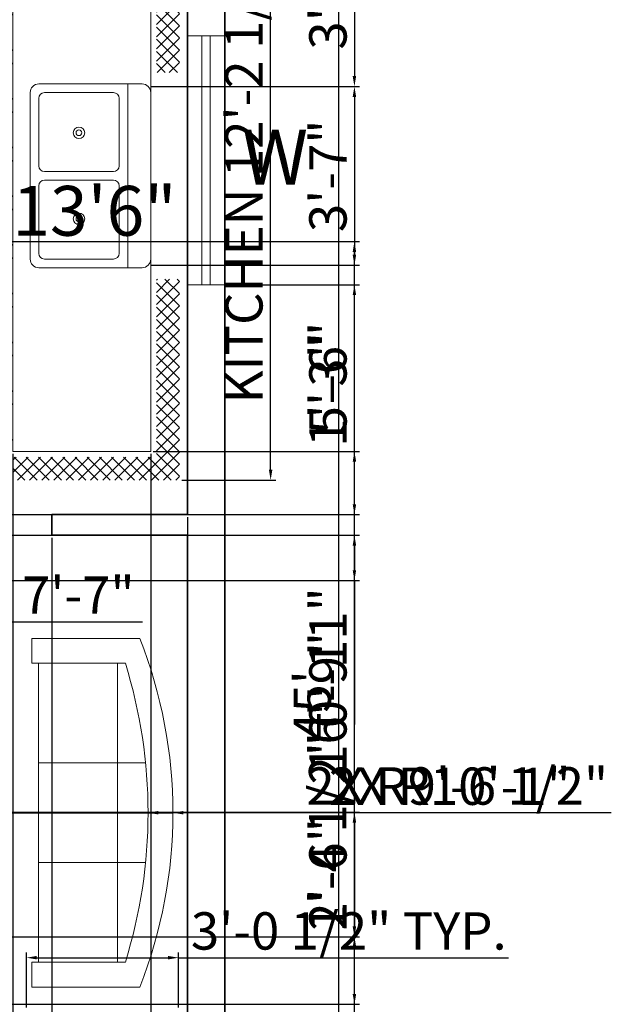
# Model space of a CAD drawing. Units: inches. Extents: x 3542 to 4275, y 1005 to 1722.
# Tile 5 of 6: x 4132 to 4275, y 1330 to 1568. Entities that reach past the tile are written whole.
import ezdxf

# ---------------------------------------------------------------- set-up
doc = ezdxf.new("R2010")
doc.units = ezdxf.units.IN
doc.layers.get('0').update_dxf_attribs({"color": 211})
for name, color, linetype, lineweight in [('A-ANNO-DIMS', 2, 'Continuous', 18), ('A-ANNO-TEXT', 7, 'Continuous', 18), ('A-AREA-IDEN', 7, 'Continuous', 25), ('A-FLOR-FIXT', 9, 'Continuous', 18), ('A-FURN', 8, 'Continuous', 18), ('A-GLAZ', 4, 'Continuous', 18), ('wall', 7, 'Continuous', 35)]:
    doc.layers.add(name, color=color, linetype=linetype, lineweight=lineweight)
doc.styles.get("Standard").update_dxf_attribs({"font": 'arial.ttf'})
doc.dimstyles.new('ISO-25', dxfattribs={"dimtxt": 9, "dimasz": 2.5, "dimexe": 1.25, "dimexo": 0.625, "dimtad": 1, "dimdec": 1, "dimlunit": 4, "dimtxsty": 'Standard', "dimcen": 2.5, "dimadec": 0, "dimazin": 0, "dimtfac": 1, "dimtdec": 1, "dimtmove": 0, "dimatfit": 3, "dimfxl": 1, "dimarcsym": 0})

# ---------------------------------------------------------------- blocks, each defined once
blk = doc.blocks.new('Kitchen Layout - 7 x 8 ft')
for p, q in [((-5, 81.32), (2.68, 89)), ((-5, 83.44), (0.56, 89)), ((-5, 85.56), (-1.56, 89)), ((-5, 87.68), (-3.68, 89)), ((-1, 84.97), (-5, 88.97)), ((1.09, 85), (-2.91, 89)), ((3.21, 85), (-0.79, 89)), ((0.81, 85), (4.81, 89)), ((5.34, 85), (1.34, 89)), ((2.93, 85), (6.93, 89)), ((7.46, 85), (3.46, 89)), ((5.05, 85), (9.05, 89)), ((9.58, 85), (5.58, 89)), ((7.17, 85), (11.17, 89)), ((11.7, 85), (7.7, 89)), ((9.29, 85), (13.29, 89)), ((13.82, 85), (9.82, 89)), ((11.41, 85), (15.41, 89)), ((15.94, 85), (11.94, 89)), ((13.53, 85), (17.53, 89)), ((18.06, 85), (14.06, 89)), ((15.65, 85), (19.65, 89)), ((20.18, 85), (16.18, 89)), ((17.78, 85), (21.78, 89)), ((22.31, 85), (18.31, 89)), ((19.9, 85), (23.9, 89)), ((24.43, 85), (20.43, 89)), ((22.02, 85), (26.02, 89)), ((26.55, 85), (22.55, 89)), ((24.14, 85), (28.14, 89)), ((28.67, 85), (24.67, 89)), ((26.26, 85), (30.26, 89)), ((30.79, 85), (26.79, 89)), ((28.38, 85), (32.38, 89)), ((32.91, 85), (28.91, 89)), ((30.5, 85), (34.5, 89)), ((35.03, 85), (31.03, 89)), ((32.63, 85), (36.63, 89)), ((37.16, 85), (33.16, 89)), ((34.75, 85), (38.75, 89)), ((39.28, 85), (35.28, 89)), ((36.87, 85), (40.87, 89)), ((41.4, 85), (37.4, 89)), ((38.99, 85), (42.99, 89)), ((43.52, 85), (39.52, 89)), ((41.11, 85), (45.11, 89)), ((45.64, 85), (41.64, 89)), ((43.23, 85), (47.23, 89)), ((47.76, 85), (43.76, 89)), ((45.35, 85), (49.35, 89)), ((49.88, 85), (45.88, 89)), ((47.47, 85), (51.47, 89)), ((52, 85), (48, 89)), ((49.6, 85), (53.6, 89)), ((54.13, 85), (50.13, 89)), ((51.72, 85), (55.72, 89)), ((56.25, 85), (52.25, 89)), ((53.84, 85), (57.84, 89)), ((58.37, 85), (54.37, 89)), ((55.96, 85), (59.96, 89)), ((60.49, 85), (56.49, 89)), ((58.08, 85), (62.08, 89)), ((62.61, 85), (58.61, 89)), ((60.2, 85), (64.2, 89)), ((64.73, 85), (60.73, 89)), ((62.32, 85), (66.32, 89)), ((66.85, 85), (62.85, 89)), ((64.45, 85), (68.45, 89)), ((68.97, 85), (64.97, 89)), ((66.57, 85), (70.57, 89)), ((71.1, 85), (67.1, 89)), ((68.69, 85), (72.69, 89)), ((73.22, 85), (69.22, 89)), ((70.81, 85), (74.81, 89)), ((75.34, 85), (71.34, 89)), ((72.93, 85), (76.93, 89)), ((77.46, 85), (73.46, 89)), ((75.05, 85), (79.05, 89)), ((79.58, 85), (75.58, 89)), ((77.17, 85), (81.17, 89)), ((81.7, 85), (77.7, 89)), ((79.29, 85), (83.29, 89)), ((83.82, 85), (79.82, 89)), ((81.42, 85), (85.42, 89)), ((85.95, 85), (81.95, 89)), ((83.54, 85), (87.54, 89)), ((88.07, 85), (84.07, 89)), ((85.66, 85), (89.66, 89)), ((90.19, 85), (86.19, 89)), ((87.78, 85), (91.78, 89)), ((92.31, 85), (88.31, 89)), ((89.9, 85), (93.9, 89)), ((94.43, 85), (90.43, 89)), ((92.02, 85), (96.02, 89)), ((96.55, 85), (92.55, 89)), ((94.14, 85), (98.14, 89)), ((101, 82.67), (94.67, 89)), ((96.27, 85), (100.27, 89)), ((101, 84.79), (96.79, 89)), ((97, 83.61), (101, 87.61)), ((101, 86.92), (98.92, 89)), ((-1, 82.85), (-5, 86.85)), ((-1, 80.73), (-5, 84.73)), ((97, 81.49), (101, 85.49)), ((101, 80.55), (97, 84.55)), ((-5, 79.19), (-1, 83.19)), ((-1, 78.61), (-5, 82.61)), ((34, 84), (96, 84)), ((34, 60), (34, 84)), ((96, 84), (96, 60)), ((97, 79.37), (101, 83.37)), ((101, 78.43), (97, 82.43)), ((-5, 77.07), (-1, 81.07)), ((74, 81), (95, 81)), ((97, 77.25), (101, 81.25)), ((-1, 76.49), (-5, 80.49)), ((-5, 74.95), (-1, 78.95)), ((101, 76.31), (97, 80.31)), ((97, 75.13), (101, 79.13)), ((-1, 74.36), (-5, 78.36)), ((101, 74.19), (97, 78.19)), ((-5, 72.83), (-1, 76.83)), ((-1, 72.24), (-5, 76.24)), ((97, 73.01), (101, 77.01)), ((101, 72.07), (97, 76.07)), ((-5, 70.71), (-1, 74.71)), ((-1, 70.12), (-5, 74.12)), ((97, 70.89), (101, 74.89)), ((101, 69.95), (97, 73.95)), ((-5, 68.59), (-1, 72.59)), ((97, 68.76), (101, 72.76)), ((-1, 68), (-5, 72)), ((-5, 66.47), (-1, 70.47)), ((101, 67.82), (97, 71.82)), ((97, 66.64), (101, 70.64)), ((-1, 65.88), (-5, 69.88)), ((101, 65.7), (97, 69.7)), ((-5, 64.35), (-1, 68.35)), ((-1, 63.76), (-5, 67.76)), ((97, 64.52), (101, 68.52)), ((101, 63.58), (97, 67.58)), ((-5, 62.22), (-1, 66.22)), ((-1, 61.64), (-5, 65.64)), ((97, 62.4), (101, 66.4)), ((101, 61.46), (97, 65.46)), ((-5, 60.1), (-1, 64.1)), ((-1, 59.52), (-5, 63.52)), ((97, 60.28), (101, 64.28)), ((-5, 57.98), (-1, 61.98)), ((100.34, 60), (97, 63.34)), ((98.84, 60), (101, 62.16)), ((-1, 57.39), (-5, 61.39)), ((98.22, 60), (97, 61.22)), ((100.96, 60), (101, 60.04)), ((-1.73, 56), (-5, 59.27)), ((-4.86, 56), (-1, 59.86)), ((10.4, 24), (45.9, 59.5)), ((18.88, 24), (54.38, 59.5)), ((27.37, 24), (62.87, 59.5)), ((33.03, 55.11), (37.41, 59.5)), ((96, 60), (34, 60)), ((35.85, 24), (71.35, 59.5)), ((76.2, 24), (40.7, 59.5)), ((84.68, 24), (49.18, 59.5)), ((93.17, 24), (57.67, 59.5)), ((61.31, 24), (96, 58.69)), ((96, 29.65), (66.15, 59.5)), ((80, 60), (80, 59)), ((82, 59), (82, 60)), ((87, 59), (87, 60)), ((89, 60), (89, 59)), ((-3.85, 56), (-5, 57.15)), ((-2.74, 56), (-1, 57.74)), ((0, 57), (33, 57)), ((67.71, 24), (33.68, 58.04)), ((44.34, 24), (77.84, 57.5)), ((52.82, 24), (86.32, 57.5)), ((96, 38.14), (76.64, 57.5)), ((96, 46.63), (85.13, 57.5)), ((96, 55.11), (93.57, 57.54)), ((0, 30.57), (24.43, 55)), ((0, 39.06), (15.94, 55)), ((0, 47.54), (7.46, 55)), ((1.91, 24), (32.91, 55)), ((33.77, 24), (2.77, 55)), ((42.26, 24), (11.26, 55)), ((50.74, 24), (19.74, 55)), ((59.23, 24), (28.23, 55)), ((31, 55), (31, 56)), ((32, 55), (31, 55)), ((32, 56), (32, 55)), ((69.79, 24), (96, 50.21)), ((25.29, 24), (0, 49.29)), ((78.28, 24), (96, 41.72)), ((16.8, 24), (0, 40.8)), ((86.76, 24), (96, 33.24)), ((8.32, 24), (0, 32.32)), ((95.25, 24), (96, 24.75)), ((-5, 21.92), (-2.92, 24)), ((-5, 19.8), (-1, 23.8)), ((-1, 19.21), (-5, 23.21)), ((-1, 21.33), (-3.67, 24)), ((-1, 23.45), (-1.55, 24)), ((0, 24), (96, 24)), ((0, 0), (0, 24)), ((96, 24), (96, 0)), ((97, 22.1), (98.9, 24)), ((97, 19.97), (101, 23.97)), ((101, 19.03), (97, 23.03)), ((101, 21.16), (98.16, 24)), ((101, 23.28), (100.28, 24)), ((-5, 17.68), (-1, 21.68)), ((-1, 17.09), (-5, 21.09)), ((97, 17.85), (101, 21.85)), ((101, 16.91), (97, 20.91)), ((-5, 15.55), (-1, 19.55)), ((-1, 14.97), (-5, 18.97)), ((97, 15.73), (101, 19.73)), ((-5, 13.43), (-1, 17.43)), ((47.25, 6.5), (47.25, 18.5)), ((48.75, 18.5), (48.75, 6.5)), ((101, 14.79), (97, 18.79)), ((97, 13.61), (101, 17.61)), ((-1, 12.85), (-5, 16.85)), ((101, 12.67), (97, 16.67)), ((97, 11.49), (101, 15.49)), ((-5, 11.31), (-1, 15.31)), ((-1, 10.73), (-5, 14.73)), ((101, 10.55), (97, 14.55)), ((-5, 9.19), (-1, 13.19)), ((-1, 8.6), (-5, 12.6)), ((97, 9.37), (101, 13.37)), ((101, 8.43), (97, 12.43)), ((-5, 7.07), (-1, 11.07)), ((-1, 6.48), (-5, 10.48)), ((97, 7.25), (101, 11.25)), ((101, 6.31), (97, 10.31)), ((-5, 4.95), (-1, 8.95)), ((97, 5.12), (101, 9.12)), ((-1, 4.36), (-5, 8.36)), ((101, 4.18), (97, 8.18)), ((97, 3), (101, 7)), ((-5, 2.83), (-1, 6.83)), ((-1, 2.24), (-5, 6.24)), ((101, 2.06), (97, 6.06)), ((-5, 0.71), (-1, 4.71)), ((-1, 0.12), (-5, 4.12)), ((64, 4), (32, 4)), ((97, 0.88), (101, 4.88)), ((101, -0.06), (97, 3.94)), ((-5, -1.42), (-1, 2.58)), ((2, -5), (-5, 2)), ((93.24, -5), (101, 2.76)), ((101, -2.18), (97, 1.82)), ((-5, -3.54), (-1, 0.46)), ((96, 0), (0, 0)), ((95.36, -5), (101, 0.64)), ((-0.12, -5), (-5, -0.12)), ((-4.34, -5), (-0.34, -1)), ((-2.22, -5), (1.78, -1)), ((-0.1, -5), (3.9, -1)), ((4.12, -5), (0.12, -1)), ((2.02, -5), (6.02, -1)), ((6.24, -5), (2.24, -1)), ((4.14, -5), (8.14, -1)), ((8.36, -5), (4.36, -1)), ((6.27, -5), (10.27, -1)), ((10.48, -5), (6.48, -1)), ((8.39, -5), (12.39, -1)), ((12.6, -5), (8.6, -1)), ((10.51, -5), (14.51, -1)), ((14.73, -5), (10.73, -1)), ((12.63, -5), (16.63, -1)), ((16.85, -5), (12.85, -1)), ((14.75, -5), (18.75, -1)), ((18.97, -5), (14.97, -1)), ((16.87, -5), (20.87, -1)), ((21.09, -5), (17.09, -1)), ((18.99, -5), (22.99, -1)), ((23.21, -5), (19.21, -1)), ((21.11, -5), (25.11, -1)), ((25.33, -5), (21.33, -1)), ((23.24, -5), (27.24, -1)), ((27.45, -5), (23.45, -1)), ((25.36, -5), (29.36, -1)), ((29.57, -5), (25.57, -1)), ((30, -3.3), (27.7, -1)), ((30, -1.18), (29.82, -1)), ((66, -2.54), (67.54, -1)), ((66, -4.66), (69.66, -1)), ((69.88, -5), (66, -1.12)), ((67.78, -5), (71.78, -1)), ((72, -5), (68, -1)), ((69.9, -5), (73.9, -1)), ((74.12, -5), (70.12, -1)), ((72.03, -5), (76.03, -1)), ((76.24, -5), (72.24, -1)), ((74.15, -5), (78.15, -1)), ((78.36, -5), (74.36, -1)), ((76.27, -5), (80.27, -1)), ((80.49, -5), (76.49, -1)), ((78.39, -5), (82.39, -1)), ((82.61, -5), (78.61, -1)), ((80.51, -5), (84.51, -1)), ((84.73, -5), (80.73, -1)), ((82.63, -5), (86.63, -1)), ((86.85, -5), (82.85, -1)), ((84.75, -5), (88.75, -1)), ((88.97, -5), (84.97, -1)), ((86.88, -5), (90.88, -1)), ((91.09, -5), (87.09, -1)), ((89, -5), (93, -1)), ((93.21, -5), (89.21, -1)), ((91.12, -5), (95.12, -1)), ((95.34, -5), (91.34, -1)), ((97.46, -5), (93.46, -1)), ((99.58, -5), (95.58, -1)), ((101, -4.3), (97, -0.3)), ((97.48, -5), (101, -1.48)), ((-2.25, -5), (-5, -2.25)), ((27.48, -5), (30, -2.48)), ((67.76, -5), (66, -3.24)), ((-4.37, -5), (-5, -4.37)), ((29.6, -5), (30, -4.6)), ((99.6, -5), (101, -3.6))]:
    blk.add_line(p, q)
for points in [[(0, 56), (0, 84), (33, 84), (33, 56)], [(74, 60), (74, 84), (95, 84), (95, 60)], [(76, 58), (76, 59), (93, 59), (93, 58)]]:
    blk.add_lwpolyline(points, close=True)
for points in [[(33.5, 21), (62.5, 21)], [(32, 1.5), (32, 19.5)], [(34.5, 19.5), (46.25, 19.5)], [(49.75, 19.5), (61.5, 19.5)], [(64, 19.5), (64, 1.5)], [(33.5, 6.5), (33.5, 18.5)], [(62.5, 18.5), (62.5, 6.5)], [(46.25, 5.5), (34.5, 5.5)], [(61.5, 5.5), (49.75, 5.5)], [(62.5, 0), (33.5, 0)]]:
    blk.add_lwpolyline(points)
for centre, radius in [((80, 75), 4), ((80, 75), 3), ((89, 75), 3), ((80, 75), 2), ((80, 75), 1), ((89, 75), 2), ((89, 75), 1), ((80, 66), 3), ((89, 66), 4), ((89, 66), 3), ((80, 66), 2), ((80, 66), 1), ((89, 66), 2), ((89, 66), 1), ((40.5, 12.5), 1), ((40.5, 12.5), 0.5), ((55.5, 12.5), 1), ((55.5, 12.5), 0.5)]:
    blk.add_circle(centre, radius)
for centre, radius, start, end in [((33.5, 19.5), 1.5, 90, 180), ((62.5, 19.5), 1.5, 0, 90), ((34.5, 18.5), 1, 90, 180), ((46.25, 18.5), 1, 0, 90), ((49.75, 18.5), 1, 90, 180), ((61.5, 18.5), 1, 0, 90), ((34.5, 6.5), 1, 180, 270), ((46.25, 6.5), 1, 270, 0), ((49.75, 6.5), 1, 180, 270), ((61.5, 6.5), 1, 270, 0), ((33.5, 1.5), 1.5, 180, 270), ((62.5, 1.5), 1.5, 270, 0)]:
    blk.add_arc(centre, radius, start, end)
blk = doc.blocks.new('Sofa - Roundback 7 ft.')
for p, q in [((-12.00002, -32.4421), (-12.00003, -6.5971)), ((11.99997, -32.4421), (11.99998, -6.5971)), ((-36.000027, -34), (-36.000027, -11.4696)), ((35.99998, -34), (35.99998, -11.4696)), ((-35.999844, -13.3819), (35.9998, -13.3819)), ((-36.000027, -32.4421), (35.99998, -32.4421))]:
    blk.add_line(p, q)
for points in [[(-36.000027, -34), (-42.000027, -34), (-42.000027, -8)], [(41.99998, -8), (41.99998, -34), (35.99998, -34)]]:
    blk.add_lwpolyline(points)
for centre, radius, start, end in [((0, -114.25), 114.25, 68.43141, 111.5686), ((-0.00001, -127.1968), 121.1968, 72.72033, 107.2797)]:
    blk.add_arc(centre, radius, start, end)
blk = doc.blocks.new('*D13')
at = {"layer": 'A-ANNO-DIMS', "color": 0, "lineweight": -2, "transparency": 16777216}
for p, q in [((4182.51, 1672.43), (4210.58, 1672.43)), ((4209.33, 1669.93), (4209.33, 1134.93)), ((4182.51, 1132.43), (4210.58, 1132.43))]:
    blk.add_line(p, q, dxfattribs=at)
at = {"layer": 'A-ANNO-DIMS', "color": 0, "transparency": 16777216}
for points in [[(4208.91, 1669.93), (4209.75, 1669.93), (4209.33, 1672.43)], [(4208.91, 1134.93), (4209.75, 1134.93), (4209.33, 1132.43)]]:
    blk.add_solid(points, dxfattribs=at)
at = {"layer": 'Defpoints', "color": 0, "transparency": 16777216}
for p in [(4181.89, 1672.43), (4181.89, 1132.43), (4209.33, 1132.43)]:
    blk.add_point(p, dxfattribs=at)
at = {"layer": 'A-ANNO-DIMS', "color": 0, "transparency": 16777216, "insert": (4204.13, 1402.43), "char_height": 9, "attachment_point": 5, "rotation": 90}
blk.add_mtext("45'", dxfattribs=at)
blk = doc.blocks.new('WIN-60IN')
for p, q in [((3.5, 60), (3.5, 0)), ((5.5, 60), (5.5, 0))]:
    blk.add_line(p, q)
blk.add_lwpolyline([(0, 60), (9, 60), (9, 0), (0, 0)], close=True)
blk = doc.blocks.new('*D24')
at = {"layer": 'A-ANNO-DIMS', "color": 0, "lineweight": -2, "transparency": 16777216}
for p, q in [((4134.07, 1329.69), (4134.07, 1342.91)), ((4170.74, 1329.69), (4170.74, 1342.91)), ((4136.57, 1341.66), (4168.24, 1341.66)), ((4170.74, 1341.66), (4250.31, 1341.66))]:
    blk.add_line(p, q, dxfattribs=at)
at = {"layer": 'A-ANNO-DIMS', "color": 0, "transparency": 16777216}
for points in [[(4136.57, 1342.08), (4136.57, 1341.24), (4134.07, 1341.66)], [(4168.24, 1342.08), (4168.24, 1341.24), (4170.74, 1341.66)]]:
    blk.add_solid(points, dxfattribs=at)
at = {"layer": 'Defpoints', "color": 0, "transparency": 16777216}
for p in [(4170.74, 1341.66), (4134.07, 1329.06), (4170.74, 1329.06)]:
    blk.add_point(p, dxfattribs=at)
at = {"layer": 'A-ANNO-DIMS', "color": 0, "transparency": 16777216, "insert": (4211.78, 1346.94), "char_height": 9, "attachment_point": 5}
blk.add_mtext('3\'-0 1/2" TYP.', dxfattribs=at)
blk = doc.blocks.new('*D27')
at = {"layer": 'A-ANNO-DIMS', "color": 0, "lineweight": -2, "transparency": 16777216}
for p, q in [((4171.57, 1603.37), (4194.19, 1603.37)), ((4192.94, 1459.24), (4192.94, 1600.87)), ((4171.57, 1456.74), (4194.19, 1456.74))]:
    blk.add_line(p, q, dxfattribs=at)
at = {"layer": 'A-ANNO-DIMS', "color": 0, "transparency": 16777216}
for points in [[(4192.52, 1600.87), (4193.36, 1600.87), (4192.94, 1603.37)], [(4192.52, 1459.24), (4193.36, 1459.24), (4192.94, 1456.74)]]:
    blk.add_solid(points, dxfattribs=at)
at = {"layer": 'Defpoints', "color": 0, "transparency": 16777216}
for p in [(4170.94, 1603.37), (4192.94, 1603.37), (4170.94, 1456.74)]:
    blk.add_point(p, dxfattribs=at)
at = {"layer": 'A-ANNO-DIMS', "color": 0, "transparency": 16777216, "insert": (4187.66, 1530.06), "char_height": 9, "attachment_point": 5, "rotation": 90}
blk.add_mtext('KITCHEN 12\'-2 1/2"', dxfattribs=at)
blk = doc.blocks.new('*D31')
at = {"layer": 'A-ANNO-DIMS', "color": 0, "lineweight": -2, "transparency": 16777216}
for p, q in [((3968.37, 1409.56), (3968.37, 1423.84)), ((4059.37, 1409.56), (4059.37, 1423.84)), ((3970.87, 1422.59), (4056.87, 1422.59)), ((4059.37, 1422.59), (4162.04, 1422.59))]:
    blk.add_line(p, q, dxfattribs=at)
at = {"layer": 'A-ANNO-DIMS', "color": 0, "transparency": 16777216}
for points in [[(3970.87, 1423.01), (3970.87, 1422.17), (3968.37, 1422.59)], [(4056.87, 1423.01), (4056.87, 1422.17), (4059.37, 1422.59)]]:
    blk.add_solid(points, dxfattribs=at)
at = {"layer": 'Defpoints', "color": 0, "transparency": 16777216}
for p in [(4059.37, 1422.59), (3968.37, 1408.94), (4059.37, 1408.94)]:
    blk.add_point(p, dxfattribs=at)
at = {"layer": 'A-ANNO-DIMS', "color": 0, "transparency": 16777216, "insert": (4111.95, 1427.87), "char_height": 9, "attachment_point": 5}
blk.add_mtext('DINING SET 7\'-7"', dxfattribs=at)
blk = doc.blocks.new('*D39')
at = {"layer": 'A-ANNO-DIMS', "color": 0, "lineweight": -2, "transparency": 16777216}
for p, q in [((4182.51, 1503.8), (4214.39, 1503.8)), ((4213.14, 1305.08), (4213.14, 1501.3)), ((4182.51, 1302.58), (4214.39, 1302.58))]:
    blk.add_line(p, q, dxfattribs=at)
at = {"layer": 'A-ANNO-DIMS', "color": 0, "transparency": 16777216}
for points in [[(4212.72, 1501.3), (4213.56, 1501.3), (4213.14, 1503.8)], [(4212.72, 1305.08), (4213.56, 1305.08), (4213.14, 1302.58)]]:
    blk.add_solid(points, dxfattribs=at)
at = {"layer": 'Defpoints', "color": 0, "transparency": 16777216}
for p in [(4181.89, 1503.8), (4213.14, 1503.8), (4181.89, 1302.58)]:
    blk.add_point(p, dxfattribs=at)
at = {"layer": 'A-ANNO-DIMS', "color": 0, "transparency": 16777216, "insert": (4207.92, 1403.19), "char_height": 9, "attachment_point": 5, "rotation": 90}
blk.add_mtext('16\'-9"', dxfattribs=at)
blk = doc.blocks.new('*D49')
at = {"layer": 'A-ANNO-DIMS', "color": 0, "lineweight": -2, "transparency": 16777216}
for p, q in [((4058.5, 1442.8), (4058.5, 1099.93)), ((4140.16, 1442.8), (4140.16, 1099.93)), ((4061, 1101.18), (4137.66, 1101.18))]:
    blk.add_line(p, q, dxfattribs=at)
at = {"layer": 'A-ANNO-DIMS', "color": 0, "transparency": 16777216}
for points in [[(4061, 1101.59), (4061, 1100.76), (4058.5, 1101.18)], [(4137.66, 1101.59), (4137.66, 1100.76), (4140.16, 1101.18)]]:
    blk.add_solid(points, dxfattribs=at)
at = {"layer": 'Defpoints', "color": 0, "transparency": 16777216}
for p in [(4058.5, 1443.43), (4140.16, 1443.43), (4140.16, 1101.18)]:
    blk.add_point(p, dxfattribs=at)
at = {"layer": 'A-ANNO-DIMS', "color": 0, "transparency": 16777216, "insert": (4099.33, 1106.46), "char_height": 9, "attachment_point": 5}
blk.add_mtext('6\'-9 1/2"', dxfattribs=at)
blk = doc.blocks.new('*D50')
at = {"layer": 'A-ANNO-DIMS', "color": 0, "lineweight": -2, "transparency": 16777216}
for p, q in [((4140.16, 1442.8), (4140.16, 1099.93)), ((4172.89, 1442.8), (4172.89, 1099.93)), ((4142.66, 1101.18), (4170.39, 1101.18)), ((4172.89, 1101.18), (4221.69, 1101.18))]:
    blk.add_line(p, q, dxfattribs=at)
at = {"layer": 'A-ANNO-DIMS', "color": 0, "transparency": 16777216}
for points in [[(4142.66, 1101.59), (4142.66, 1100.76), (4140.16, 1101.18)], [(4170.39, 1101.59), (4170.39, 1100.76), (4172.89, 1101.18)]]:
    blk.add_solid(points, dxfattribs=at)
at = {"layer": 'Defpoints', "color": 0, "transparency": 16777216}
for p in [(4140.16, 1443.43), (4172.89, 1443.43), (4172.89, 1101.18)]:
    blk.add_point(p, dxfattribs=at)
at = {"layer": 'A-ANNO-DIMS', "color": 0, "transparency": 16777216, "insert": (4198.54, 1106.46), "char_height": 9, "attachment_point": 5}
blk.add_mtext('2\'-8 1/2"', dxfattribs=at)
blk = doc.blocks.new('*D53')
at = {"layer": 'A-ANNO-DIMS', "color": 0, "lineweight": -2, "transparency": 16777216}
for p, q in [((4130.83, 1463.03), (4130.83, 1099.93)), ((4164.03, 1463.03), (4164.03, 1099.93)), ((4133.33, 1101.18), (4161.53, 1101.18))]:
    blk.add_line(p, q, dxfattribs=at)
at = {"layer": 'A-ANNO-DIMS', "color": 0, "transparency": 16777216}
for points in [[(4133.33, 1101.59), (4133.33, 1100.76), (4130.83, 1101.18)], [(4161.53, 1101.59), (4161.53, 1100.76), (4164.03, 1101.18)]]:
    blk.add_solid(points, dxfattribs=at)
at = {"layer": 'Defpoints', "color": 0, "transparency": 16777216}
for p in [(4130.83, 1463.65), (4164.03, 1463.65), (4164.03, 1101.18)]:
    blk.add_point(p, dxfattribs=at)
at = {"layer": 'A-ANNO-DIMS', "color": 0, "transparency": 16777216, "insert": (4147.43, 1106.4), "char_height": 9, "attachment_point": 5}
blk.add_mtext('2\'-9"', dxfattribs=at)
blk = doc.blocks.new('*D56')
at = {"layer": 'A-ANNO-DIMS', "color": 0, "lineweight": -2, "transparency": 16777216}
for p, q in [((4213.14, 1463.65), (4213.14, 1490.48)), ((4164.65, 1463.65), (4214.39, 1463.65)), ((4213.14, 1450.93), (4213.14, 1461.15)), ((4173.51, 1448.43), (4214.39, 1448.43))]:
    blk.add_line(p, q, dxfattribs=at)
at = {"layer": 'A-ANNO-DIMS', "color": 0, "transparency": 16777216}
for points in [[(4212.72, 1461.15), (4213.56, 1461.15), (4213.14, 1463.65)], [(4212.72, 1450.93), (4213.56, 1450.93), (4213.14, 1448.43)]]:
    blk.add_solid(points, dxfattribs=at)
at = {"layer": 'Defpoints', "color": 0, "transparency": 16777216}
for p in [(4164.03, 1463.65), (4213.14, 1463.65), (4172.89, 1448.43)]:
    blk.add_point(p, dxfattribs=at)
at = {"layer": 'A-ANNO-DIMS', "color": 0, "transparency": 16777216, "insert": (4207.92, 1478.32), "char_height": 9, "attachment_point": 5, "rotation": 90}
blk.add_mtext('1\'-3"', dxfattribs=at)
blk = doc.blocks.new('*D57')
at = {"layer": 'A-ANNO-DIMS', "color": 0, "lineweight": -2, "transparency": 16777216}
for p, q in [((4164.03, 1463.03), (4164.03, 1099.93)), ((4172.89, 1447.8), (4172.89, 1099.93)), ((4164.03, 1101.18), (4136.35, 1101.18)), ((4170.39, 1101.18), (4166.53, 1101.18))]:
    blk.add_line(p, q, dxfattribs=at)
at = {"layer": 'A-ANNO-DIMS', "color": 0, "transparency": 16777216}
for points in [[(4166.53, 1101.59), (4166.53, 1100.76), (4164.03, 1101.18)], [(4170.39, 1101.59), (4170.39, 1100.76), (4172.89, 1101.18)]]:
    blk.add_solid(points, dxfattribs=at)
at = {"layer": 'Defpoints', "color": 0, "transparency": 16777216}
for p in [(4164.03, 1463.65), (4172.89, 1448.43), (4164.03, 1101.18)]:
    blk.add_point(p, dxfattribs=at)
at = {"layer": 'A-ANNO-DIMS', "color": 0, "transparency": 16777216, "insert": (4148.94, 1106.4), "char_height": 9, "attachment_point": 5}
blk.add_mtext('0\'-9"', dxfattribs=at)
blk = doc.blocks.new('*D58')
at = {"layer": 'A-ANNO-DIMS', "color": 0, "lineweight": -2, "transparency": 16777216}
for p, q in [((4164.65, 1596.46), (4214.39, 1596.46)), ((4213.14, 1593.96), (4213.14, 1554.08)), ((4164.04, 1551.58), (4214.39, 1551.58))]:
    blk.add_line(p, q, dxfattribs=at)
at = {"layer": 'A-ANNO-DIMS', "color": 0, "transparency": 16777216}
for points in [[(4212.72, 1593.96), (4213.56, 1593.96), (4213.14, 1596.46)], [(4212.72, 1554.08), (4213.56, 1554.08), (4213.14, 1551.58)]]:
    blk.add_solid(points, dxfattribs=at)
at = {"layer": 'Defpoints', "color": 0, "transparency": 16777216}
for p in [(4164.03, 1596.46), (4163.42, 1551.58), (4213.14, 1551.58)]:
    blk.add_point(p, dxfattribs=at)
at = {"layer": 'A-ANNO-DIMS', "color": 0, "transparency": 16777216, "insert": (4207.92, 1574.02), "char_height": 9, "attachment_point": 5, "rotation": 90}
blk.add_mtext('3\'-9"', dxfattribs=at)
blk = doc.blocks.new('*D59')
at = {"layer": 'A-ANNO-DIMS', "color": 0, "lineweight": -2, "transparency": 16777216}
for p, q in [((4164.04, 1551.58), (4214.39, 1551.58)), ((4213.14, 1549.08), (4213.14, 1511.03)), ((4164.04, 1508.53), (4214.39, 1508.53))]:
    blk.add_line(p, q, dxfattribs=at)
at = {"layer": 'A-ANNO-DIMS', "color": 0, "transparency": 16777216}
for points in [[(4212.72, 1549.08), (4213.56, 1549.08), (4213.14, 1551.58)], [(4212.72, 1511.03), (4213.56, 1511.03), (4213.14, 1508.53)]]:
    blk.add_solid(points, dxfattribs=at)
at = {"layer": 'Defpoints', "color": 0, "transparency": 16777216}
for p in [(4163.42, 1551.58), (4163.42, 1508.53), (4213.14, 1508.53)]:
    blk.add_point(p, dxfattribs=at)
at = {"layer": 'A-ANNO-DIMS', "color": 0, "transparency": 16777216, "insert": (4207.92, 1530.06), "char_height": 9, "attachment_point": 5, "rotation": 90}
blk.add_mtext('3\'-7"', dxfattribs=at)
blk = doc.blocks.new('*D64')
at = {"layer": 'A-ANNO-DIMS', "color": 0, "lineweight": -2, "transparency": 16777216}
for p, q in [((3741.01, 1376.72), (4214.39, 1376.72)), ((4213.14, 1374.22), (4213.14, 1349.22)), ((3741.01, 1346.72), (4214.39, 1346.72))]:
    blk.add_line(p, q, dxfattribs=at)
at = {"layer": 'A-ANNO-DIMS', "color": 0, "transparency": 16777216}
for points in [[(4212.72, 1374.22), (4213.56, 1374.22), (4213.14, 1376.72)], [(4212.72, 1349.22), (4213.56, 1349.22), (4213.14, 1346.72)]]:
    blk.add_solid(points, dxfattribs=at)
at = {"layer": 'Defpoints', "color": 0, "transparency": 16777216}
for p in [(3740.38, 1376.72), (3740.38, 1346.72), (4213.14, 1346.72)]:
    blk.add_point(p, dxfattribs=at)
at = {"layer": 'A-ANNO-DIMS', "color": 0, "transparency": 16777216, "insert": (4207.92, 1361.72), "char_height": 9, "attachment_point": 5, "rotation": 90}
blk.add_mtext('2\'-6"', dxfattribs=at)
blk = doc.blocks.new('*D66')
at = {"layer": 'A-ANNO-DIMS', "color": 0, "lineweight": -2, "transparency": 16777216}
for p, q in [((3735.51, 1443.43), (4214.39, 1443.43)), ((4213.14, 1440.93), (4213.14, 1435.03)), ((3735.95, 1432.53), (4214.39, 1432.53)), ((4213.14, 1432.53), (4213.14, 1397.86))]:
    blk.add_line(p, q, dxfattribs=at)
at = {"layer": 'A-ANNO-DIMS', "color": 0, "transparency": 16777216}
for points in [[(4212.72, 1440.93), (4213.56, 1440.93), (4213.14, 1443.43)], [(4212.72, 1435.03), (4213.56, 1435.03), (4213.14, 1432.53)]]:
    blk.add_solid(points, dxfattribs=at)
at = {"layer": 'Defpoints', "color": 0, "transparency": 16777216}
for p in [(3734.89, 1443.43), (3735.32, 1432.53), (4213.14, 1432.53)]:
    blk.add_point(p, dxfattribs=at)
at = {"layer": 'A-ANNO-DIMS', "color": 0, "transparency": 16777216, "insert": (4207.92, 1413.94), "char_height": 9, "attachment_point": 5, "rotation": 90}
blk.add_mtext('0\'-11"', dxfattribs=at)
blk = doc.blocks.new('*D67')
at = {"layer": 'A-ANNO-DIMS', "color": 0, "lineweight": -2, "transparency": 16777216}
for p, q in [((4213.14, 1346.72), (4213.14, 1394.52)), ((3741.01, 1346.72), (4214.39, 1346.72)), ((4213.14, 1332.93), (4213.14, 1344.22)), ((3740.51, 1330.43), (4214.39, 1330.43))]:
    blk.add_line(p, q, dxfattribs=at)
at = {"layer": 'A-ANNO-DIMS', "color": 0, "transparency": 16777216}
for points in [[(4212.72, 1344.22), (4213.56, 1344.22), (4213.14, 1346.72)], [(4212.72, 1332.93), (4213.56, 1332.93), (4213.14, 1330.43)]]:
    blk.add_solid(points, dxfattribs=at)
at = {"layer": 'Defpoints', "color": 0, "transparency": 16777216}
for p in [(3740.38, 1346.72), (4213.14, 1346.72), (3739.89, 1330.43)]:
    blk.add_point(p, dxfattribs=at)
at = {"layer": 'A-ANNO-DIMS', "color": 0, "transparency": 16777216, "insert": (4207.86, 1371.87), "char_height": 9, "attachment_point": 5, "rotation": 90}
blk.add_mtext('1\'-4 1/2"', dxfattribs=at)
blk = doc.blocks.new('*D73')
at = {"layer": 'A-ANNO-DIMS', "color": 0, "lineweight": -2, "transparency": 16777216}
for p, q in [((3836.51, 1514.23), (4214.39, 1514.23)), ((4213.14, 1450.93), (4213.14, 1511.73)), ((3836.51, 1448.43), (4214.39, 1448.43))]:
    blk.add_line(p, q, dxfattribs=at)
at = {"layer": 'A-ANNO-DIMS', "color": 0, "transparency": 16777216}
for points in [[(4212.72, 1511.73), (4213.56, 1511.73), (4213.14, 1514.23)], [(4212.72, 1450.93), (4213.56, 1450.93), (4213.14, 1448.43)]]:
    blk.add_solid(points, dxfattribs=at)
at = {"layer": 'Defpoints', "color": 0, "transparency": 16777216}
for p in [(3835.89, 1514.23), (4213.14, 1514.23), (3835.89, 1448.43)]:
    blk.add_point(p, dxfattribs=at)
at = {"layer": 'A-ANNO-DIMS', "color": 0, "transparency": 16777216, "insert": (4207.92, 1481.33), "char_height": 9, "attachment_point": 5, "rotation": 90}
blk.add_mtext('5\'-6"', dxfattribs=at)
blk = doc.blocks.new('*D74')
at = {"layer": 'A-ANNO-DIMS', "color": 0, "lineweight": -2, "transparency": 16777216}
for p, q in [((4042.19, 1376.59), (4163.39, 1376.59)), ((4266.24, 1376.59), (4165.89, 1376.59))]:
    blk.add_line(p, q, dxfattribs=at)
at = {"layer": 'A-ANNO-DIMS', "color": 0, "transparency": 16777216}
blk.add_solid([(4165.89, 1377.01), (4165.89, 1376.18), (4163.39, 1376.59)], dxfattribs=at)
at = {"layer": 'Defpoints', "color": 0, "transparency": 16777216}
for p in [(4042.19, 1376.59), (4163.39, 1376.59)]:
    blk.add_point(p, dxfattribs=at)
at = {"layer": 'A-ANNO-DIMS', "color": 0, "transparency": 16777216, "insert": (4236.11, 1381.81), "char_height": 9, "attachment_point": 5, "rotation": 359.9999}
blk.add_mtext('2X R10\'-1"', dxfattribs=at)
blk = doc.blocks.new('*D75')
at = {"layer": 'A-ANNO-DIMS', "color": 0, "lineweight": -2, "transparency": 16777216}
for p, q in [((4055.14, 1376.59), (4169.39, 1376.59)), ((4275.07, 1376.59), (4171.89, 1376.59))]:
    blk.add_line(p, q, dxfattribs=at)
at = {"layer": 'A-ANNO-DIMS', "color": 0, "transparency": 16777216}
blk.add_solid([(4171.89, 1377.01), (4171.89, 1376.18), (4169.39, 1376.59)], dxfattribs=at)
at = {"layer": 'Defpoints', "color": 0, "transparency": 16777216}
for p in [(4055.14, 1376.59), (4169.39, 1376.59)]:
    blk.add_point(p, dxfattribs=at)
at = {"layer": 'A-ANNO-DIMS', "color": 0, "transparency": 16777216, "insert": (4237.94, 1381.87), "char_height": 9, "attachment_point": 5, "rotation": 359.9999}
blk.add_mtext('2X R9\'-6 1/2"', dxfattribs=at)

msp = doc.modelspace()

# ---------------------------------------------------------------- linework, layer by layer
at = {"layer": 'wall'}
for p, q in [((4181.89, 1672.43), (4181.89, 1132.43)), ((4172.89, 1610.43), (4172.89, 1448.43)), ((4140.16, 1443.43), (4140.16, 1448.43)), ((4140.16, 1448.43), (4172.89, 1448.43)), ((4140.16, 1443.43), (4172.89, 1443.43)), ((4140.16, 1443.43), (4172.89, 1443.43)), ((4172.89, 1443.43), (4172.89, 1141.43)), ((4172.89, 1443.43), (4172.89, 1335.43))]:
    msp.add_line(p, q, dxfattribs=at)

# ---------------------------------------------------------------- block references
at = {"layer": 'A-FLOR-FIXT', "xscale": 1.383356761737284, "yscale": 1.383356761737284, "zscale": 1.383356761737284, "rotation": 90}
msp.add_blockref('Kitchen Layout - 7 x 8 ft', (4164.03, 1463.65), dxfattribs=at)
at = {"layer": 'A-FURN', "rotation": 270}
msp.add_blockref('Sofa - Roundback 7 ft.', (4169.39, 1376.59), dxfattribs=at)
at = {"layer": 'A-GLAZ'}
msp.add_blockref('WIN-60IN', (4172.89, 1503.8), dxfattribs=at)

# ---------------------------------------------------------------- texts
at = {"layer": 'A-ANNO-TEXT'}
msp.add_text('W', height=13.28, dxfattribs=at).set_placement((4186.08, 1527.93))
at = {"layer": 'A-AREA-IDEN'}
msp.add_text('12\'8"X13\'6"', height=12, dxfattribs=at).set_placement((4081.72, 1515.62))

# ---------------------------------------------------------------- dimensions: what is measured, and where the dimension line sits
at = {"layer": 'A-ANNO-DIMS'}
for base, p1, p2, override, picture, middle in [((4209.33, 1132.43), (4181.89, 1672.43), (4181.89, 1132.43), {"dimclrd": 0, "dimclre": 0, "dimclrt": 0}, '*D13', (4204.13, 1402.43)), ((4213.14, 1551.58), (4164.03, 1596.46), (4163.42, 1551.58), {"dimdec": 1, "dimlfac": 1, "dimrnd": 0, "dimzin": 1, "dimdsep": 46, "dimlunit": 4, "dimfrac": 2}, '*D58', (4207.92, 1574.02)), ((4213.1394, 1508.5293), (4163.4187, 1551.5812), (4163.4187, 1508.5293), {"dimdec": 1, "dimlfac": 1, "dimrnd": 0, "dimzin": 1, "dimdsep": 46, "dimlunit": 4, "dimfrac": 2}, '*D59', (4207.9161, 1530.0553)), ((4213.14, 1514.23), (3835.89, 1448.43), (3835.89, 1514.23), {"dimdec": 1, "dimlfac": 1, "dimrnd": 0, "dimzin": 1, "dimdsep": 46, "dimlunit": 4, "dimfrac": 2}, '*D73', (4207.92, 1481.33)), ((4213.14, 1503.8), (4181.89, 1302.58), (4181.89, 1503.8), {"dimdec": 1, "dimlfac": 1, "dimrnd": 0, "dimzin": 1, "dimdsep": 46, "dimlunit": 4, "dimfrac": 2}, '*D39', (4207.92, 1403.19)), ((4213.14, 1463.65), (4172.89, 1448.43), (4164.03, 1463.65), {"dimdec": 1, "dimlfac": 1, "dimrnd": 0, "dimzin": 1, "dimdsep": 46, "dimlunit": 4, "dimfrac": 2}, '*D56', (4207.92, 1478.32)), ((4213.14, 1432.53), (3734.89, 1443.43), (3735.32, 1432.53), {"dimdec": 1, "dimlfac": 1, "dimrnd": 0, "dimzin": 1, "dimdsep": 46, "dimlunit": 4, "dimfrac": 2}, '*D66', (4207.92, 1413.94)), ((4213.14, 1346.72), (3739.89, 1330.43), (3740.38, 1346.72), {"dimdec": 1, "dimlfac": 1, "dimrnd": 0, "dimzin": 1, "dimdsep": 46, "dimlunit": 4, "dimfrac": 2}, '*D67', (4207.86, 1371.87)), ((4213.14, 1346.72), (3740.38, 1376.72), (3740.38, 1346.72), {"dimdec": 1, "dimlfac": 1, "dimrnd": 0, "dimzin": 1, "dimdsep": 46, "dimlunit": 4, "dimfrac": 2}, '*D64', (4207.92, 1361.72))]:
    dim = msp.add_linear_dim(base=base, p1=p1, p2=p2, angle=90, dimstyle='ISO-25', override=override, dxfattribs=at)
    dim.commit()
    dim.dimension.update_dxf_attribs({"geometry": picture, "text_midpoint": middle})
dim = msp.add_linear_dim(base=(4192.94, 1603.37), p1=(4170.94, 1456.74), p2=(4170.94, 1603.37), angle=90, text='KITCHEN <>', dimstyle='ISO-25', override={"dimdec": 1, "dimlfac": 1, "dimrnd": 0, "dimzin": 1, "dimdsep": 46, "dimlunit": 4, "dimfrac": 2}, dxfattribs=at)
dim.commit()
dim.dimension.update_dxf_attribs({"geometry": '*D27', "text_midpoint": (4187.66, 1530.06)})
for base, p1, p2, picture, middle in [((4164.03, 1101.18), (4130.83, 1463.65), (4164.03, 1463.65), '*D53', (4147.43, 1106.4)), ((4164.03, 1101.18), (4172.89, 1448.43), (4164.03, 1463.65), '*D57', (4148.94, 1106.4)), ((4140.16, 1101.18), (4058.5, 1443.43), (4140.16, 1443.43), '*D49', (4099.33, 1106.46)), ((4172.89, 1101.18), (4140.16, 1443.43), (4172.89, 1443.43), '*D50', (4198.54, 1106.46))]:
    dim = msp.add_linear_dim(base=base, p1=p1, p2=p2, dimstyle='ISO-25', override={"dimdec": 1, "dimlfac": 1, "dimrnd": 0, "dimzin": 1, "dimdsep": 46, "dimlunit": 4, "dimfrac": 2}, dxfattribs=at)
    dim.commit()
    dim.dimension.update_dxf_attribs({"geometry": picture, "text_midpoint": middle})
for base, p1, p2, text, picture, middle in [((4059.37, 1422.59), (3968.37, 1408.94), (4059.37, 1408.94), 'DINING SET <>', '*D31', (4111.95, 1427.87)), ((4170.74, 1341.66), (4134.07, 1329.06), (4170.74, 1329.06), '<> TYP.', '*D24', (4211.78, 1346.94))]:
    dim = msp.add_linear_dim(base=base, p1=p1, p2=p2, text=text, dimstyle='ISO-25', override={"dimdec": 1, "dimlfac": 1, "dimrnd": 0, "dimzin": 1, "dimdsep": 46, "dimlunit": 4, "dimfrac": 2}, dxfattribs=at)
    dim.commit()
    dim.dimension.update_dxf_attribs({"geometry": picture, "text_midpoint": middle})
for center, mpoint, picture, middle in [((4055.140656, 1376.593166), (4169.390656, 1376.593), '*D75', (4237.940656, 1376.5929004)), ((4042.19, 1376.59), (4163.39, 1376.59), '*D74', (4236.11, 1376.59))]:
    dim = msp.add_radius_dim(center=center, mpoint=mpoint, text='2X <>', dimstyle='ISO-25', override={"dimdec": 1, "dimlfac": 1, "dimrnd": 0, "dimzin": 1, "dimdsep": 46, "dimlunit": 4, "dimfrac": 2}, dxfattribs=at)
    dim.commit()
    dim.dimension.update_dxf_attribs({"geometry": picture, "text_midpoint": middle, "dimtype": 164})

doc.saveas('drawing.dxf')
